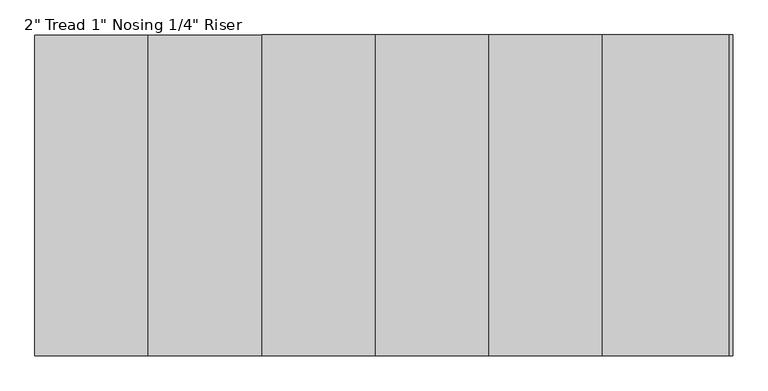
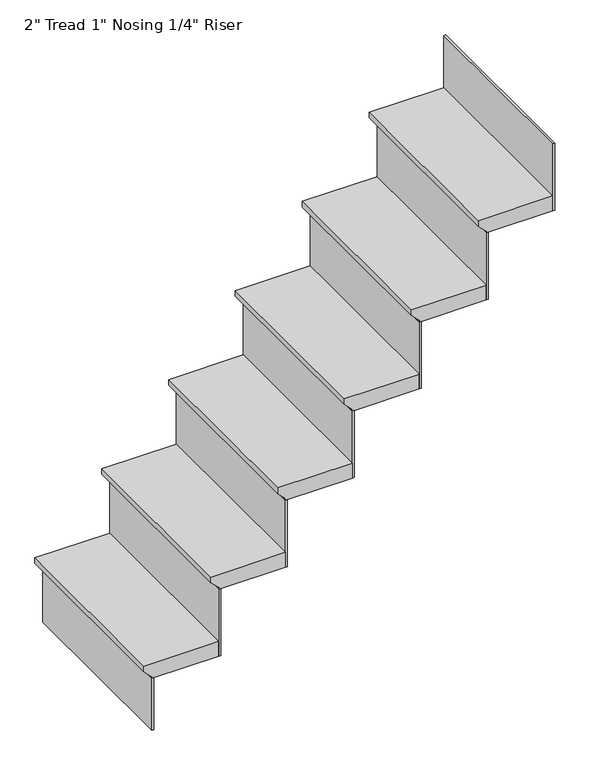
"""IFC4 building model written with IfcOpenShell, lengths in millimetres: stair flight geometry."""

from ifc_helpers import new_model, si_unit, origin, place, context, project, spatial, faceted_brep, source, transform, mapped, element, save


def stair_flight_b3ddc6eb(model_context):
    return source(origin(), model_context, "Body", "Brep", [
        faceted_brep([(-5028.1409298, -3848.0779636, 6610.35), (-5028.1409298, -3848.0779636, 6629.4), (-5028.1409298, -3238.4779636, 6629.4), (-5028.1409298, -3238.4779636, 6610.35), (-5002.7409298, -3848.0779636, 6584.95), (-5002.7409298, -3238.4779636, 6584.95), (-4786.8409298, -3848.0779636, 6629.4), (-4786.8409298, -3238.4779636, 6629.4), (-5002.7409298, -3238.4779636, 6578.6), (-4786.8409298, -3238.4779636, 6578.6), (-4786.8409298, -3848.0779636, 6578.6), (-5002.7409298, -3848.0779636, 6578.6)], [[[0, 1, 2, 3]], [[4, 0, 3, 5]], [[2, 1, 6, 7]], [[8, 9, 10, 11]], [[2, 7, 9, 8, 5, 3]], [[8, 11, 4, 5]], [[6, 1, 0, 4, 11, 10]], [[7, 6, 10, 9]]]),
        faceted_brep([(-5002.7409298, -3848.0779636, 6578.6), (-5002.7409298, -3848.0779636, 6400.8), (-4996.3909298, -3848.0779636, 6400.8), (-4996.3909298, -3848.0779636, 6578.6), (-5002.7409298, -3238.4779636, 6578.6), (-4996.3909298, -3238.4779636, 6578.6), (-4996.3909298, -3238.4779636, 6400.8), (-5002.7409298, -3238.4779636, 6400.8)], [[[0, 1, 2, 3]], [[4, 5, 6, 7]], [[1, 0, 4, 7]], [[2, 1, 7, 6]], [[3, 2, 6, 5]], [[0, 3, 5, 4]]]),
        faceted_brep([(-4786.8409298, -3848.0779636, 6807.2), (-4786.8409298, -3848.0779636, 6578.6), (-4780.4909298, -3848.0779636, 6578.6), (-4780.4909298, -3848.0779636, 6807.2), (-4786.8409298, -3238.4779636, 6807.2), (-4780.4909298, -3238.4779636, 6807.2), (-4780.4909298, -3238.4779636, 6578.6), (-4786.8409298, -3238.4779636, 6578.6)], [[[0, 1, 2, 3]], [[4, 5, 6, 7]], [[1, 0, 4, 7]], [[2, 1, 7, 6]], [[3, 2, 6, 5]], [[0, 3, 5, 4]]]),
        faceted_brep([(-4812.2409298, -3238.4779636, 6858.0), (-4812.2409298, -3848.0779636, 6858.0), (-4570.9409298, -3848.0779636, 6858.0), (-4570.9409298, -3238.4779636, 6858.0), (-4786.8409298, -3238.4779636, 6807.2), (-4570.9409298, -3238.4779636, 6807.2), (-4570.9409298, -3848.0779636, 6807.2), (-4786.8409298, -3848.0779636, 6807.2), (-4786.8409298, -3238.4779636, 6813.55), (-4812.2409298, -3238.4779636, 6838.95), (-4786.8409298, -3848.0779636, 6813.55), (-4812.2409298, -3848.0779636, 6838.95)], [[[0, 1, 2, 3]], [[4, 5, 6, 7]], [[0, 3, 5, 4, 8, 9]], [[4, 7, 10, 8]], [[2, 1, 11, 10, 7, 6]], [[3, 2, 6, 5]], [[11, 1, 0, 9]], [[10, 11, 9, 8]]]),
        faceted_brep([(-4570.9409298, -3848.0779636, 7035.8), (-4570.9409298, -3848.0779636, 6807.2), (-4564.5909298, -3848.0779636, 6807.2), (-4564.5909298, -3848.0779636, 7035.8), (-4570.9409298, -3238.4779636, 7035.8), (-4564.5909298, -3238.4779636, 7035.8), (-4564.5909298, -3238.4779636, 6807.2), (-4570.9409298, -3238.4779636, 6807.2)], [[[0, 1, 2, 3]], [[4, 5, 6, 7]], [[1, 0, 4, 7]], [[2, 1, 7, 6]], [[3, 2, 6, 5]], [[0, 3, 5, 4]]]),
        faceted_brep([(-4596.3409298, -3238.4779636, 7086.6), (-4596.3409298, -3848.0779636, 7086.6), (-4355.0409298, -3848.0779636, 7086.6), (-4355.0409298, -3238.4779636, 7086.6), (-4570.9409298, -3238.4779636, 7035.8), (-4355.0409298, -3238.4779636, 7035.8), (-4355.0409298, -3848.0779636, 7035.8), (-4570.9409298, -3848.0779636, 7035.8), (-4570.9409298, -3238.4779636, 7042.15), (-4596.3409298, -3238.4779636, 7067.55), (-4570.9409298, -3848.0779636, 7042.15), (-4596.3409298, -3848.0779636, 7067.55)], [[[0, 1, 2, 3]], [[4, 5, 6, 7]], [[0, 3, 5, 4, 8, 9]], [[4, 7, 10, 8]], [[2, 1, 11, 10, 7, 6]], [[3, 2, 6, 5]], [[11, 1, 0, 9]], [[10, 11, 9, 8]]]),
        faceted_brep([(-4355.0409298, -3848.0779636, 7264.4), (-4355.0409298, -3848.0779636, 7035.8), (-4348.6909298, -3848.0779636, 7035.8), (-4348.6909298, -3848.0779636, 7264.4), (-4355.0409298, -3238.4779636, 7264.4), (-4348.6909298, -3238.4779636, 7264.4), (-4348.6909298, -3238.4779636, 7035.8), (-4355.0409298, -3238.4779636, 7035.8)], [[[0, 1, 2, 3]], [[4, 5, 6, 7]], [[1, 0, 4, 7]], [[2, 1, 7, 6]], [[3, 2, 6, 5]], [[0, 3, 5, 4]]]),
        faceted_brep([(-4380.4409298, -3238.4779636, 7315.2), (-4380.4409298, -3848.0779636, 7315.2), (-4139.1409298, -3848.0779636, 7315.2), (-4139.1409298, -3238.4779636, 7315.2), (-4355.0409298, -3238.4779636, 7264.4), (-4139.1409298, -3238.4779636, 7264.4), (-4139.1409298, -3848.0779636, 7264.4), (-4355.0409298, -3848.0779636, 7264.4), (-4355.0409298, -3238.4779636, 7270.75), (-4380.4409298, -3238.4779636, 7296.15), (-4355.0409298, -3848.0779636, 7270.75), (-4380.4409298, -3848.0779636, 7296.15)], [[[0, 1, 2, 3]], [[4, 5, 6, 7]], [[0, 3, 5, 4, 8, 9]], [[4, 7, 10, 8]], [[2, 1, 11, 10, 7, 6]], [[3, 2, 6, 5]], [[11, 1, 0, 9]], [[10, 11, 9, 8]]]),
        faceted_brep([(-4139.1409298, -3848.0779636, 7493.0), (-4139.1409298, -3848.0779636, 7264.4), (-4132.7909298, -3848.0779636, 7264.4), (-4132.7909298, -3848.0779636, 7493.0), (-4139.1409298, -3238.4779636, 7493.0), (-4132.7909298, -3238.4779636, 7493.0), (-4132.7909298, -3238.4779636, 7264.4), (-4139.1409298, -3238.4779636, 7264.4)], [[[0, 1, 2, 3]], [[4, 5, 6, 7]], [[1, 0, 4, 7]], [[2, 1, 7, 6]], [[3, 2, 6, 5]], [[0, 3, 5, 4]]]),
        faceted_brep([(-4164.5409298, -3238.4779636, 7543.8), (-4164.5409298, -3848.0779636, 7543.8), (-3923.2409298, -3848.0779636, 7543.8), (-3923.2409298, -3238.4779636, 7543.8), (-4139.1409298, -3238.4779636, 7493.0), (-3923.2409298, -3238.4779636, 7493.0), (-3923.2409298, -3848.0779636, 7493.0), (-4139.1409298, -3848.0779636, 7493.0), (-4139.1409298, -3238.4779636, 7499.35), (-4164.5409298, -3238.4779636, 7524.75), (-4139.1409298, -3848.0779636, 7499.35), (-4164.5409298, -3848.0779636, 7524.75)], [[[0, 1, 2, 3]], [[4, 5, 6, 7]], [[0, 3, 5, 4, 8, 9]], [[4, 7, 10, 8]], [[2, 1, 11, 10, 7, 6]], [[3, 2, 6, 5]], [[11, 1, 0, 9]], [[10, 11, 9, 8]]]),
        faceted_brep([(-3707.3409298, -3848.0779636, 7950.2), (-3707.3409298, -3848.0779636, 7721.6), (-3700.9909298, -3848.0779636, 7721.6), (-3700.9909298, -3848.0779636, 7950.2), (-3707.3409298, -3238.4779636, 7950.2), (-3700.9909298, -3238.4779636, 7950.2), (-3700.9909298, -3238.4779636, 7721.6), (-3707.3409298, -3238.4779636, 7721.6)], [[[0, 1, 2, 3]], [[4, 5, 6, 7]], [[1, 0, 4, 7]], [[2, 1, 7, 6]], [[3, 2, 6, 5]], [[0, 3, 5, 4]]]),
        faceted_brep([(-3923.2409298, -3848.0779636, 7721.6), (-3923.2409298, -3848.0779636, 7493.0), (-3916.8909298, -3848.0779636, 7493.0), (-3916.8909298, -3848.0779636, 7721.6), (-3923.2409298, -3238.4779636, 7721.6), (-3916.8909298, -3238.4779636, 7721.6), (-3916.8909298, -3238.4779636, 7493.0), (-3923.2409298, -3238.4779636, 7493.0)], [[[0, 1, 2, 3]], [[4, 5, 6, 7]], [[1, 0, 4, 7]], [[2, 1, 7, 6]], [[3, 2, 6, 5]], [[0, 3, 5, 4]]]),
        faceted_brep([(-3707.3409298, -3238.4779636, 7772.4), (-3732.7409298, -3238.4779636, 7772.4), (-3948.6409298, -3238.4779636, 7772.4), (-3948.6409298, -3848.0779636, 7772.4), (-3707.3409298, -3848.0779636, 7772.4), (-3732.7409298, -3238.4779636, 7721.6), (-3707.3409298, -3238.4779636, 7721.6), (-3707.3409298, -3848.0779636, 7721.6), (-3923.2409298, -3848.0779636, 7721.6), (-3923.2409298, -3238.4779636, 7721.6), (-3923.2409298, -3238.4779636, 7727.95), (-3948.6409298, -3238.4779636, 7753.35), (-3923.2409298, -3848.0779636, 7727.95), (-3948.6409298, -3848.0779636, 7753.35)], [[[0, 1, 2, 3, 4]], [[5, 6, 7, 8, 9]], [[1, 0, 6, 5]], [[2, 1, 5, 9, 10, 11]], [[9, 8, 12, 10]], [[4, 3, 13, 12, 8, 7]], [[0, 4, 7, 6]], [[13, 3, 2, 11]], [[12, 13, 11, 10]]]),
    ])


if __name__ == "__main__":
    model = new_model("IFC4")
    model_context = context("Model", 3, world=origin())
    ifc_project = project(units=[si_unit("LENGTHUNIT", "METRE", prefix="MILLI")], contexts=[model_context])
    site = spatial("IfcSite", under=ifc_project)
    building = spatial("IfcBuilding", under=site)
    placement = place(None, origin())
    stair_flight_shape = stair_flight_b3ddc6eb(model_context)
    element("IfcStairFlight", 1, ObjectType="2\" Tread 1\" Nosing 1/4\" Riser", at=placement, inside=building, context=model_context, shape_type="MappedRepresentation", body=[
        mapped(stair_flight_shape, transform((0.0, 0.0, 0.0), x_axis=(1.0, 0.0, 0.0), y_axis=(0.0, 1.0, 0.0), z_axis=(0.0, 0.0, 1.0))),
    ])
    save(model, "model.ifc")
